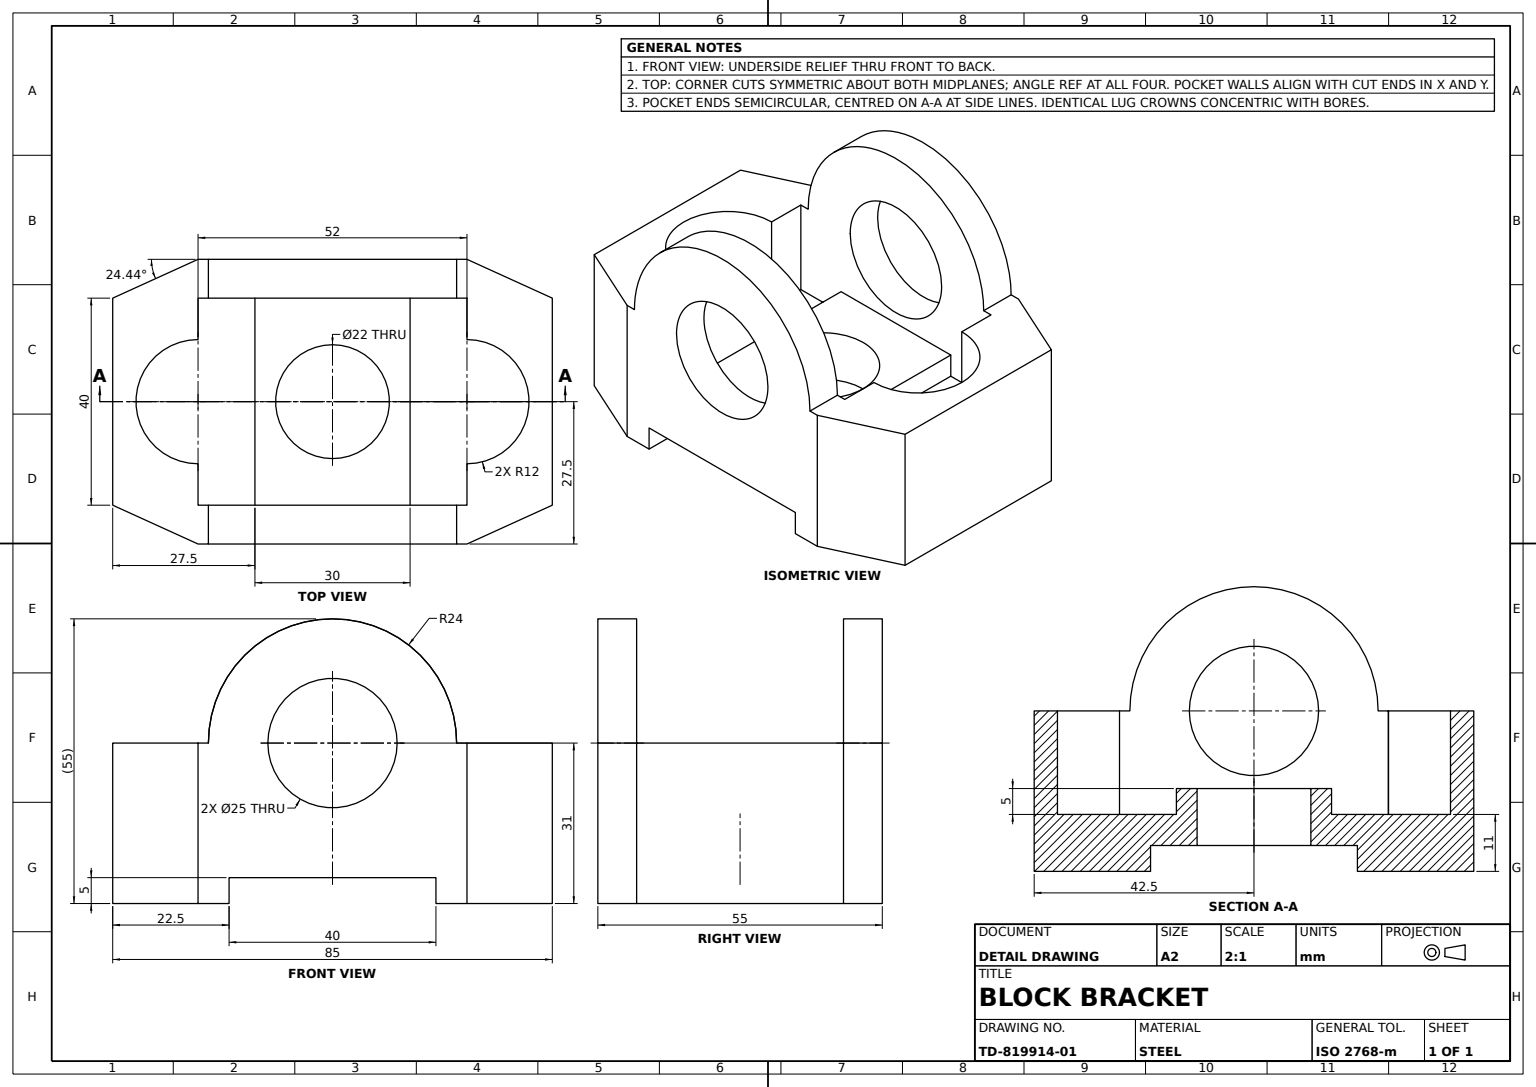
from build123d import *

# Parameters (mm, degrees)
BASE_BLOCK_DEPTH           = 31
LUG_A_DEPTH                = 7.5
LUG_START                  = -7.5
LUG_A_WEB_DEPTH            = 7.5
BORE_25_PROFILE_R          = 12.5
BORE_25_DEPTH              = 89.635489506
LUG_B_BASE_DEPTH           = 11
LUG_B_PROFILE_W            = 30
LUG_B_PROFILE_H            = 40
LUG_B_DEPTH                = 5
BORE_22_REACH              = 65.902
BORE_22_PROFILE_R          = 11
RELIEF_SLOT_40X5_REACH     = 90.635
RELIEF_SLOT_40X5_PROFILE_W = 40
RELIEF_SLOT_40X5_PROFILE_H = 5


with BuildPart() as part:
    # Base Block Profile → Base Block (new body)
    with BuildSketch(Plane(origin=(0, 0, 0), x_dir=(1, 0, 0), z_dir=(0, 1, 0))):
        Polygon((-26, 27.5), (26, 27.5), (42.5, 20), (42.5, -20), (26, -27.5), (-26, -27.5), (-42.5, -20), (-42.5, 20), align=None)
        with BuildLine():
            Line((-26, 20), (26, 20))
            Line((26, 20), (26, 12))
            ThreePointArc((26, 12), (38, 0), (26, -12))
            Line((26, -12), (26, -20))
            Line((26, -20), (-26, -20))
            Line((-26, -20), (-26, -12))
            ThreePointArc((-26, -12), (-38, 0), (-26, 12))
            Line((-26, 12), (-26, 20))
        make_face(mode=Mode.SUBTRACT)
    extrude(amount=BASE_BLOCK_DEPTH)

    # Lug A Profile → Lug A (add)
    with BuildSketch(Plane.XY.offset(27.5)):
        with BuildLine():
            Line((-24, 31), (24, 31))
            ThreePointArc((24, 31), (0, 55), (-24, 31))
        make_face()
    extrude(amount=-LUG_A_DEPTH)

    # Lug A Web Profile → Lug A Web (add)
    with BuildSketch(Plane(origin=(0, 0, -27.5), x_dir=(-1, 0, 0), z_dir=(0, 0, -1)).offset(LUG_START)):
        with BuildLine():
            Line((-24, 31), (24, 31))
            ThreePointArc((24, 31), (0, 55), (-24, 31))
        make_face()
    extrude(amount=LUG_A_WEB_DEPTH)

    # Bore _25 Profile → Bore _25 (cut, through all)
    with BuildSketch(Plane.XY.offset(27.5)):
        with Locations((0, 31)):
            Circle(BORE_25_PROFILE_R)
    extrude(amount=-BORE_25_DEPTH, mode=Mode.SUBTRACT)

    # Lug B Base Profile → Lug B Base (add)
    with BuildSketch(Plane(origin=(0, 0, 0), x_dir=(1, 0, 0), z_dir=(0, 1, 0))):
        Polygon((42.5, 20), (26, 27.5), (-26, 27.5), (-42.5, 20), (-42.5, -20), (-26, -27.5), (26, -27.5), (42.5, -20), align=None)
    extrude(amount=LUG_B_BASE_DEPTH)

    # Lug B Profile → Lug B (add)
    with BuildSketch(Plane(origin=(0, 11, 0), x_dir=(1, 0, 0), z_dir=(0, 1, 0))):
        Rectangle(LUG_B_PROFILE_W, LUG_B_PROFILE_H)
    extrude(amount=LUG_B_DEPTH)

    # Bore _22 Profile → Bore _22 (cut, up to next)
    with BuildSketch(Plane(origin=(0, 16, 0), x_dir=(1, 0, 0), z_dir=(0, 1, 0)), mode=Mode.PRIVATE) as bore_22_sk1:
        with Locations(Location((0, 0, 0), (0, 0, 270))):
            Circle(BORE_22_PROFILE_R)
    bore_22_tool1 = extrude(bore_22_sk1.sketch, amount=-BORE_22_REACH, mode=Mode.PRIVATE) & part.part
    add(bore_22_tool1.solids().sort_by_distance((0, 16, 0))[0], mode=Mode.SUBTRACT)

    # Relief Slot 40x5 Profile → Relief Slot 40x5 (cut, up to next)
    with BuildSketch(Plane.XY.offset(27.5), mode=Mode.PRIVATE) as relief_slot_40x5_sk1:
        with Locations((0, 2.5)):
            Rectangle(RELIEF_SLOT_40X5_PROFILE_W, RELIEF_SLOT_40X5_PROFILE_H)
    relief_slot_40x5_tool1 = extrude(relief_slot_40x5_sk1.sketch, amount=-RELIEF_SLOT_40X5_REACH, mode=Mode.PRIVATE) & part.part
    add(relief_slot_40x5_tool1.solids().sort_by_distance((0, 2.5, 27.5))[0], mode=Mode.SUBTRACT)


solid = part.part
